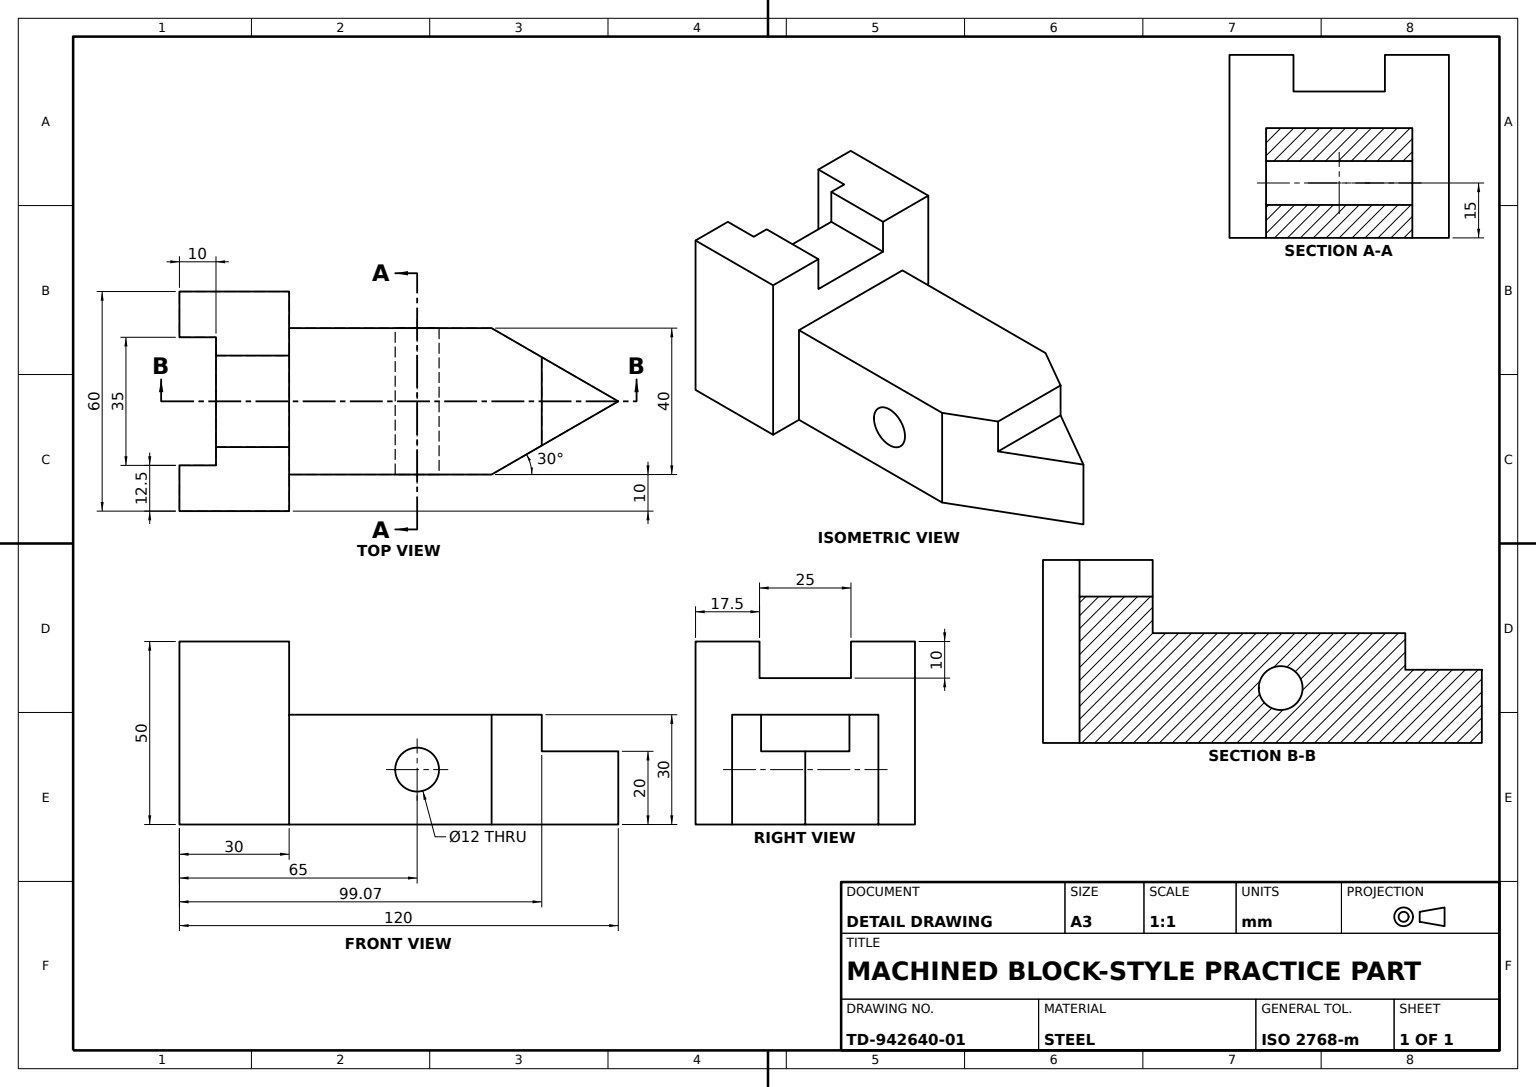
from build123d import *

# Parameters (mm, degrees)
BASE_BLOCK_SKETCH_W        = 30
BASE_BLOCK_SKETCH_H        = 50
BASE_BLOCK_DEPTH           = 30
THROUGH_SLOT_SKETCH_W      = 10
THROUGH_SLOT_SKETCH_H      = 35
THROUGH_SLOT_DEPTH         = 60
STEP_NOTCH_SKETCH_W        = 25
STEP_NOTCH_SKETCH_H        = 10
STEP_NOTCH_DEPTH           = 60
NOSE_BOSS_SKETCH_W         = 40
NOSE_BOSS_SKETCH_H         = 30
NOSE_BOSS_DEPTH            = 90
CORNER_CUT_SKETCH_R        = 6
CORNER_CUT_DEPTH           = 60
NOSE_TAPER_30DEG_CUT_DEPTH = 60
SIDE_POCKET_SKETCH_W       = 22.012832553
SIDE_POCKET_SKETCH_H       = 24.1626403
SIDE_POCKET_10MM_DEPTH     = 10
NOSE_PROFILE_CUT_DEPTH     = 30


with BuildPart() as part:
    # Base Block Sketch → Base Block (new, symmetric)
    with BuildSketch(Plane.XY):
        with Locations((15, 25)):
            Rectangle(BASE_BLOCK_SKETCH_W, BASE_BLOCK_SKETCH_H)
    extrude(amount=BASE_BLOCK_DEPTH, both=True)

    # Through Slot Sketch → Through Slot (cut)
    with BuildSketch(Plane(origin=(0, 50, 0), x_dir=(1, 0, 0), z_dir=(0, 1, 0))):
        with Locations((5, 0)):
            Rectangle(THROUGH_SLOT_SKETCH_W, THROUGH_SLOT_SKETCH_H)
    extrude(amount=-THROUGH_SLOT_DEPTH, mode=Mode.SUBTRACT)

    # Step Notch Sketch → Step Notch (cut)
    with BuildSketch(Plane(origin=(30, 0, 0), x_dir=(0, 0, -1), z_dir=(1, 0, 0))):
        with Locations((0, 45)):
            Rectangle(STEP_NOTCH_SKETCH_W, STEP_NOTCH_SKETCH_H)
    extrude(amount=-STEP_NOTCH_DEPTH, mode=Mode.SUBTRACT)

    # Nose Boss Sketch → Nose Boss (add)
    with BuildSketch(Plane(origin=(30, 0, 0), x_dir=(0, 0, -1), z_dir=(1, 0, 0))):
        with Locations((0, 15)):
            Rectangle(NOSE_BOSS_SKETCH_W, NOSE_BOSS_SKETCH_H)
    extrude(amount=NOSE_BOSS_DEPTH)

    # Corner Cut Sketch → Corner Cut (cut)
    with BuildSketch(Plane.XY.offset(20)):
        with Locations((65, 15)):
            Circle(CORNER_CUT_SKETCH_R)
    extrude(amount=-CORNER_CUT_DEPTH, mode=Mode.SUBTRACT)

    # Nose Taper 30deg Sketch → Nose Taper 30deg Cut (cut)
    with BuildSketch(Plane(origin=(0, 30, 0), x_dir=(1, 0, 0), z_dir=(0, 1, 0))):
        Polygon((99.074539678, -20), (120, -20), (120, 0), (99.074539678, -12.08132015), align=None)
        Polygon((99.074539678, 12.08132015), (120, 0), (120, 20), (99.074539678, 20), align=None)
    extrude(amount=-NOSE_TAPER_30DEG_CUT_DEPTH, mode=Mode.SUBTRACT)

    # Side Pocket Sketch → Side Pocket 10mm (cut)
    with BuildSketch(Plane(origin=(0, 30, 0), x_dir=(1, 0, 0), z_dir=(0, 1, 0))):
        with Locations((110.080955955, 0)):
            Rectangle(SIDE_POCKET_SKETCH_W, SIDE_POCKET_SKETCH_H)
    extrude(amount=-SIDE_POCKET_10MM_DEPTH, mode=Mode.SUBTRACT)

    # Nose Profile Sketch → Nose Profile Cut (cut)
    with BuildSketch(Plane(origin=(0, 30, 0), x_dir=(1, 0, 0), z_dir=(0, 1, 0))):
        Polygon((85.358983849, 20), (99.074539678, 12.08132015), (99.074539678, 20), align=None)
        Polygon((99.074539678, -20), (99.074539678, -12.08132015), (85.358983849, -20), align=None)
    extrude(amount=-NOSE_PROFILE_CUT_DEPTH, mode=Mode.SUBTRACT)


solid = part.part
